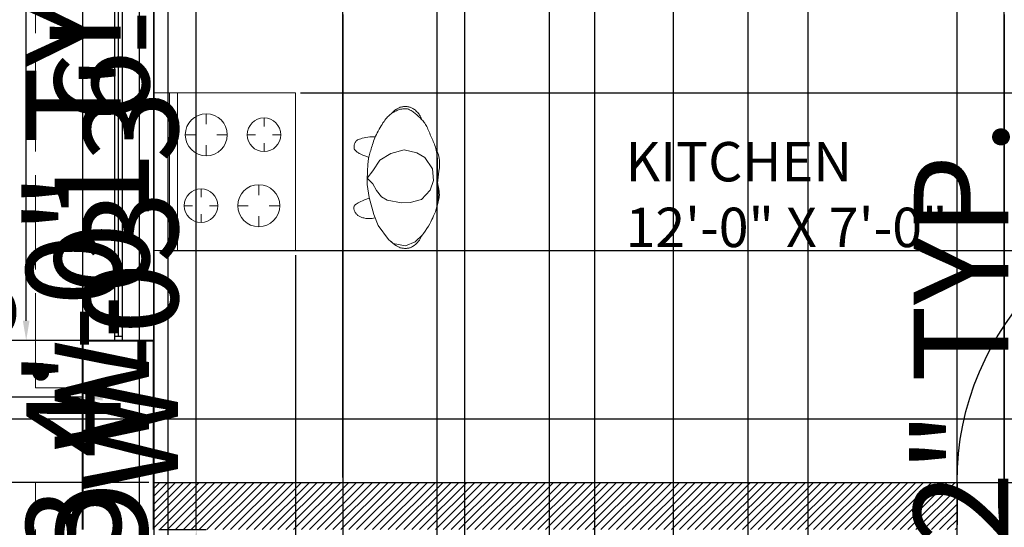
# Model space of a CAD drawing. Units: inches. Extents: x 2386 to 3029, y 792 to 1465.
# Tile 7 of 12: x 2463 to 2588, y 1140 to 1205. Entities that reach past the tile are written whole.
import ezdxf

# ---------------------------------------------------------------- set-up
doc = ezdxf.new("R2010")
doc.units = ezdxf.units.IN
doc.linetypes.add('ACAD_ISO02W100', pattern=[15, 12, -3])
for name, color, linetype, lineweight in [('A-AREA-IDEN', 4, 'Continuous', 25), ('A-DIMS', 1, 'Continuous', 18), ('A-DOOR', 2, 'Continuous', 25), ('A-EQPM', 8, 'Continuous', 18), ('A-FLOR-CASE', 6, 'Continuous', 18), ('A-FURN-ENTG', 8, 'Continuous', 13), ('A-WALL-EXT', 7, 'Continuous', 40), ('A-WALL-INT', 9, 'Continuous', 30), ('A-WALL-PATT', 9, 'Continuous', 13), ('A-WINDOW', 4, 'Continuous', 25), ('A-WINDOW-OVHD', 4, 'ACAD_ISO02W100', 18)]:
    doc.layers.add(name, color=color, linetype=linetype, lineweight=lineweight)
doc.styles.add('ATT', font='romans.shx')
doc.styles.get("Standard").update_dxf_attribs({"font": 'arial.ttf'})
doc.dimstyles.new('ISO-25', dxfattribs={"dimtxt": 12, "dimasz": 2.5, "dimexe": 1.25, "dimexo": 0.625, "dimtad": 1, "dimlunit": 4, "dimtxsty": 'Standard', "dimcen": 2.5, "dimadec": 0, "dimazin": 0, "dimtfac": 1, "dimtmove": 0, "dimatfit": 3, "dimfxl": 1, "dimarcsym": 0})

# ---------------------------------------------------------------- blocks, each defined once
blk = doc.blocks.new('*U14')
for p, q in [((-40, 0), (-40, 6)), ((0, 0), (0, 6))]:
    blk.add_line(p, q)
blk.add_lwpolyline([(0, 0), (0, -40), (-1.75, -40), (-1.75, 0)], close=True)
blk.add_arc((0, 0), 40, 180, 270)
blk = doc.blocks.new('11PRNG01')
at = {"color": 0, "linetype": 'ByBlock'}
for p, q in [((0, 30), (27, 30)), ((0, 0), (0, 30)), ((3, 0), (3, 30)), ((4.5, 0), (4.5, 30)), ((27, 30), (27, 0)), ((10, 26), (10, 24)), ((21, 25.2), (21, 23.6)), ((6, 22), (8, 22)), ((14, 22), (12, 22)), ((17.8, 22), (19.4, 22)), ((24.2, 22), (22.6, 22)), ((10, 18), (10, 20)), ((21, 18.8), (21, 20.4)), ((9, 11.7), (9, 10.1)), ((20, 12.5), (20, 10.5)), ((5.8, 8.5), (7.4, 8.5)), ((12.2, 8.5), (10.6, 8.5)), ((16, 8.5), (18, 8.5)), ((24, 8.5), (22, 8.5)), ((9, 5.3), (9, 6.9)), ((20, 4.5), (20, 6.5)), ((27, 0), (0, 0))]:
    blk.add_line(p, q, dxfattribs=at)
for centre, radius in [((10, 22), 4), ((21, 22), 3.2), ((9, 8.5), 3.2), ((20, 8.5), 4)]:
    blk.add_circle(centre, radius, dxfattribs=at)
at = {"color": 0, "linetype": 'ByBlock', "style": 'ATT'}
for tag, p, flags in [('ITEM', (0, -11), 3), ('ROOM_NUMBER', (0, -20), 1), ('DEPTH', (0, -29), 3), ('WIDTH', (0, -38), 3)]:
    blk.add_attdef(tag, p, '', height=6, dxfattribs=dict(at, flags=flags))
blk = doc.blocks.new('PERSON-STANDING-PLAN')
for p, q in [((4.11, 9.95), (4.28, 10.02)), ((4.28, 10.02), (4.45, 10.1)), ((4.45, 10.1), (4.62, 10.18)), ((4.62, 10.18), (4.79, 10.25)), ((4.79, 10.25), (4.96, 10.31)), ((4.96, 10.31), (5.14, 10.38)), ((5.14, 10.38), (5.33, 10.43)), ((5.33, 10.43), (5.53, 10.48)), ((5.48, 10.5), (5.36, 10.44)), ((5.69, 10.59), (5.48, 10.5)), ((5.53, 10.48), (5.74, 10.51)), ((5.91, 10.67), (5.69, 10.59)), ((5.74, 10.51), (5.95, 10.55)), ((6.13, 10.74), (5.91, 10.67)), ((5.95, 10.55), (6.17, 10.57)), ((6.35, 10.79), (6.13, 10.74)), ((6.17, 10.57), (6.39, 10.59)), ((6.57, 10.84), (6.35, 10.79)), ((6.39, 10.59), (6.61, 10.61)), ((6.79, 10.87), (6.57, 10.84)), ((6.61, 10.61), (6.83, 10.62)), ((6.99, 10.89), (6.79, 10.87)), ((6.83, 10.62), (7.05, 10.63)), ((7.18, 10.9), (6.99, 10.89)), ((7.05, 10.63), (7.26, 10.64)), ((7.38, 10.9), (7.18, 10.9)), ((7.26, 10.64), (7.47, 10.65)), ((7.57, 10.88), (7.38, 10.9)), ((7.47, 10.65), (7.68, 10.65)), ((7.78, 10.87), (7.57, 10.88)), ((7.68, 10.65), (7.87, 10.65)), ((7.99, 10.84), (7.78, 10.87)), ((7.87, 10.65), (8.06, 10.65)), ((9.39, 10.13), (7.91, 9.98)), ((8.22, 10.82), (7.99, 10.84)), ((8.06, 10.65), (8.23, 10.65)), ((9.71, 10.64), (8.22, 10.82)), ((8.23, 10.65), (8.39, 10.65)), ((8.39, 10.65), (8.54, 10.64)), ((8.54, 10.64), (8.67, 10.64)), ((8.67, 10.64), (8.78, 10.63)), ((8.78, 10.63), (8.89, 10.62)), ((8.89, 10.62), (8.98, 10.61)), ((8.98, 10.61), (9.08, 10.6)), ((9.08, 10.6), (9.16, 10.59)), ((9.16, 10.59), (9.25, 10.59)), ((9.25, 10.59), (9.35, 10.59)), ((9.35, 10.59), (9.44, 10.59)), ((10.63, 9.72), (9.39, 10.13)), ((9.44, 10.59), (9.55, 10.6)), ((9.55, 10.6), (9.66, 10.61)), ((9.9, 10.69), (9.56, 10.61)), ((9.66, 10.61), (9.78, 10.62)), ((9.78, 10.62), (9.9, 10.63)), ((10.22, 10.76), (9.9, 10.69)), ((9.9, 10.63), (10.03, 10.64)), ((10.03, 10.64), (10.16, 10.66)), ((10.16, 10.66), (10.3, 10.67)), ((10.5, 10.81), (10.22, 10.76)), ((10.3, 10.67), (10.45, 10.68)), ((10.45, 10.68), (10.61, 10.7)), ((10.76, 10.84), (10.5, 10.81)), ((10.61, 10.7), (10.76, 10.71)), ((10.99, 10.86), (10.76, 10.84)), ((10.76, 10.71), (10.92, 10.71)), ((10.92, 10.71), (11.09, 10.72)), ((11.2, 10.87), (10.99, 10.86)), ((11.09, 10.72), (11.25, 10.72)), ((11.4, 10.86), (11.2, 10.87)), ((11.25, 10.72), (11.41, 10.72)), ((11.58, 10.84), (11.4, 10.86)), ((11.41, 10.72), (11.57, 10.71)), ((11.57, 10.71), (11.73, 10.7)), ((11.76, 10.81), (11.58, 10.84)), ((11.73, 10.7), (11.89, 10.68)), ((11.93, 10.77), (11.76, 10.81)), ((11.89, 10.68), (12.04, 10.67)), ((12.11, 10.73), (11.93, 10.77)), ((12.04, 10.67), (12.19, 10.64)), ((12.29, 10.67), (12.11, 10.73)), ((12.19, 10.64), (12.34, 10.62)), ((12.48, 10.61), (12.29, 10.67)), ((12.34, 10.62), (12.48, 10.59)), ((12.68, 10.55), (12.48, 10.61)), ((12.48, 10.59), (12.63, 10.56)), ((12.63, 10.56), (12.77, 10.53)), ((12.91, 10.49), (12.68, 10.55)), ((12.77, 10.53), (12.91, 10.49)), ((12.91, 10.49), (13.05, 10.45)), ((13.17, 10.43), (12.91, 10.49)), ((13.05, 10.45), (13.2, 10.41)), ((13.2, 10.41), (13.35, 10.36)), ((13.35, 10.36), (13.51, 10.3)), ((13.51, 10.3), (13.69, 10.22)), ((13.69, 10.22), (13.89, 10.14)), ((13.89, 10.14), (14.11, 10.04)), ((14.11, 10.04), (14.35, 9.93)), ((1.69, 8.66), (1.79, 8.76)), ((1.79, 8.76), (1.9, 8.85)), ((1.9, 8.85), (2.01, 8.94)), ((2.01, 8.94), (2.13, 9.02)), ((2.13, 9.02), (2.26, 9.11)), ((2.26, 9.11), (2.39, 9.19)), ((2.39, 9.19), (2.54, 9.27)), ((2.54, 9.27), (2.7, 9.35)), ((2.7, 9.35), (2.86, 9.42)), ((2.86, 9.42), (3.04, 9.5)), ((3.04, 9.5), (3.21, 9.57)), ((3.21, 9.57), (3.39, 9.65)), ((3.39, 9.65), (3.58, 9.72)), ((3.58, 9.72), (3.76, 9.79)), ((3.76, 9.79), (3.94, 9.87)), ((3.94, 9.87), (4.11, 9.95)), ((6.48, 9.01), (5.88, 8.02)), ((7.91, 9.98), (6.48, 9.01)), ((11.79, 8.58), (10.63, 9.72)), ((14.35, 9.93), (14.61, 9.79)), ((14.61, 9.79), (14.89, 9.64)), ((14.89, 9.64), (15.18, 9.47)), ((15.18, 9.47), (15.49, 9.28)), ((15.49, 9.28), (15.8, 9.07)), ((15.8, 9.07), (16.12, 8.84)), ((16.12, 8.84), (16.44, 8.59)), ((0.25, 7.51), (0.2, 7.42)), ((0.32, 7.61), (0.25, 7.51)), ((0.39, 7.71), (0.32, 7.61)), ((0.48, 7.82), (0.39, 7.71)), ((0.57, 7.92), (0.48, 7.82)), ((0.67, 8.02), (0.57, 7.92)), ((0.6, 7.41), (0.68, 7.53)), ((0.77, 8.12), (0.67, 8.02)), ((0.68, 7.53), (0.76, 7.64)), ((0.76, 7.64), (0.85, 7.75)), ((0.87, 8.21), (0.77, 8.12)), ((0.85, 7.75), (0.94, 7.85)), ((0.97, 8.29), (0.87, 8.21)), ((0.94, 7.85), (1.03, 7.96)), ((1.08, 8.36), (0.97, 8.29)), ((1.03, 7.96), (1.12, 8.07)), ((1.17, 8.42), (1.08, 8.36)), ((1.12, 8.07), (1.21, 8.17)), ((1.26, 8.47), (1.17, 8.42)), ((1.21, 8.17), (1.3, 8.27)), ((1.35, 8.51), (1.26, 8.47)), ((1.3, 8.27), (1.39, 8.37)), ((1.43, 8.54), (1.35, 8.51)), ((1.39, 8.37), (1.49, 8.47)), ((1.49, 8.56), (1.43, 8.54)), ((1.55, 8.58), (1.49, 8.56)), ((1.49, 8.47), (1.59, 8.57)), ((1.59, 8.59), (1.55, 8.58)), ((1.59, 8.57), (1.69, 8.66)), ((1.62, 8.6), (1.59, 8.59)), ((5.88, 8.02), (5.48, 6.38)), ((12.18, 7.14), (11.79, 8.58)), ((16.26, 8.74), (17.17, 7.78)), ((16.44, 8.59), (16.61, 8.53)), ((16.61, 8.53), (16.77, 8.45)), ((16.77, 8.45), (16.94, 8.35)), ((16.94, 8.35), (17.1, 8.23)), ((17.1, 8.23), (17.25, 8.1)), ((17.17, 7.78), (17.68, 6.58)), ((17.25, 8.1), (17.38, 7.96)), ((17.38, 7.96), (17.51, 7.82)), ((17.51, 7.82), (17.61, 7.69)), ((17.61, 7.69), (17.7, 7.56)), ((17.7, 7.56), (17.78, 7.45)), ((0.01, 6.79), (0, 6.7)), ((0, 6.7), (0, 6.61)), ((0, 6.61), (0, 6.52)), ((0, 6.52), (0, 6.42)), ((0, 6.42), (0.01, 6.33)), ((0.02, 6.88), (0.01, 6.79)), ((0.01, 6.33), (0.02, 6.22)), ((0.04, 6.97), (0.02, 6.88)), ((0.06, 7.06), (0.04, 6.97)), ((0.08, 7.15), (0.06, 7.06)), ((0.11, 7.23), (0.08, 7.15)), ((0.15, 7.32), (0.11, 7.23)), ((0.2, 7.42), (0.15, 7.32)), ((0.28, 6.52), (0.29, 6.66)), ((0.29, 6.38), (0.28, 6.52)), ((0.29, 6.66), (0.31, 6.8)), ((0.3, 6.24), (0.29, 6.38)), ((0.31, 6.8), (0.35, 6.93)), ((0.35, 6.93), (0.4, 7.06)), ((0.4, 7.06), (0.46, 7.18)), ((0.46, 7.18), (0.52, 7.3)), ((0.52, 7.3), (0.6, 7.41)), ((5.48, 6.38), (5.95, 4.72)), ((12.22, 6.07), (12.18, 7.14)), ((17.68, 6.58), (17.36, 5.01)), ((17.78, 7.45), (17.84, 7.34)), ((17.84, 7.34), (17.88, 7.24)), ((17.88, 7.24), (17.92, 7.15)), ((17.92, 7.15), (17.95, 7.06)), ((17.95, 7.06), (17.97, 6.97)), ((17.97, 6.97), (17.98, 6.88)), ((17.98, 6.88), (17.99, 6.79)), ((17.99, 6.33), (17.98, 6.22)), ((17.99, 6.79), (18, 6.7)), ((18, 6.42), (17.99, 6.33)), ((18, 6.7), (18.01, 6.61)), ((18.01, 6.52), (18, 6.42)), ((18.01, 6.61), (18.01, 6.52)), ((0.02, 6.22), (0.04, 6.12)), ((0.04, 6.12), (0.06, 6)), ((0.06, 6), (0.1, 5.88)), ((0.1, 5.88), (0.15, 5.75)), ((0.15, 5.75), (0.23, 5.6)), ((0.23, 5.6), (0.33, 5.43)), ((0.32, 6.09), (0.3, 6.24)), ((0.35, 5.95), (0.32, 6.09)), ((0.33, 5.43), (0.48, 5.23)), ((0.39, 5.81), (0.35, 5.95)), ((0.43, 5.68), (0.39, 5.81)), ((0.48, 5.55), (0.43, 5.68)), ((0.53, 5.42), (0.48, 5.55)), ((0.48, 5.23), (0.67, 5.01)), ((0.58, 5.3), (0.53, 5.42)), ((0.64, 5.19), (0.58, 5.3)), ((0.7, 5.07), (0.64, 5.19)), ((0.67, 5.01), (0.91, 4.75)), ((0.77, 4.96), (0.7, 5.07)), ((11.9, 4.25), (12.22, 6.07)), ((17.36, 5.01), (16.88, 4.4)), ((17.54, 5.23), (17.37, 5)), ((17.68, 5.42), (17.54, 5.23)), ((17.78, 5.6), (17.68, 5.42)), ((17.86, 5.75), (17.78, 5.6)), ((17.91, 5.88), (17.86, 5.75)), ((17.94, 6), (17.91, 5.88)), ((17.96, 6.12), (17.94, 6)), ((17.98, 6.22), (17.96, 6.12)), ((0.85, 4.85), (0.77, 4.96)), ((0.93, 4.74), (0.85, 4.85)), ((1.01, 4.63), (0.93, 4.74)), ((1.1, 4.52), (1.01, 4.63)), ((1.21, 4.41), (1.1, 4.52)), ((1.32, 4.3), (1.21, 4.41)), ((1.44, 4.19), (1.32, 4.3)), ((1.57, 4.08), (1.44, 4.19)), ((1.72, 3.96), (1.57, 4.08)), ((1.88, 3.84), (1.72, 3.96)), ((2.06, 3.71), (1.88, 3.84)), ((5.95, 4.72), (6.81, 3.29)), ((11.44, 3.53), (11.9, 4.25)), ((16.88, 4.4), (15.08, 3.08)), ((17.37, 5), (17.14, 4.74)), ((2.26, 3.59), (2.06, 3.71)), ((2.46, 3.46), (2.26, 3.59)), ((2.67, 3.34), (2.46, 3.46)), ((2.89, 3.21), (2.67, 3.34)), ((3.11, 3.09), (2.89, 3.21)), ((3.33, 2.98), (3.11, 3.09)), ((3.56, 2.87), (3.33, 2.98)), ((3.77, 2.77), (3.56, 2.87)), ((3.99, 2.68), (3.77, 2.77)), ((3.86, 2.7), (3.84, 2.5)), ((4.2, 2.6), (3.99, 2.68)), ((4.4, 2.52), (4.2, 2.6)), ((4.6, 2.45), (4.4, 2.52)), ((6.81, 3.29), (8.17, 2.41)), ((9.82, 2.41), (10.66, 2.88)), ((10.66, 2.88), (11.44, 3.53)), ((13.68, 2.54), (11.53, 1.95)), ((15.08, 3.08), (13.68, 2.54)), ((14.17, 2.51), (14.14, 2.7)), ((14.19, 2.34), (14.17, 2.51)), ((3.84, 2.5), (3.84, 2.27)), ((3.84, 2.27), (3.86, 2.03)), ((3.86, 2.03), (3.89, 1.79)), ((3.89, 1.79), (3.93, 1.54)), ((3.93, 1.54), (3.98, 1.3)), ((3.98, 1.3), (4.03, 1.08)), ((4.8, 2.38), (4.6, 2.45)), ((5, 2.32), (4.8, 2.38)), ((5.19, 2.26), (5, 2.32)), ((5.38, 2.2), (5.19, 2.26)), ((5.56, 2.15), (5.38, 2.2)), ((5.74, 2.09), (5.56, 2.15)), ((5.92, 2.05), (5.74, 2.09)), ((6.09, 2), (5.92, 2.05)), ((6.25, 1.96), (6.09, 2)), ((6.17, 1.17), (6.26, 1.39)), ((6.41, 1.92), (6.25, 1.96)), ((6.26, 1.39), (6.36, 1.65)), ((6.36, 1.65), (6.46, 1.91)), ((6.55, 1.89), (6.41, 1.92)), ((6.7, 1.86), (6.55, 1.89)), ((6.85, 1.83), (6.7, 1.86)), ((7.04, 1.81), (6.85, 1.83)), ((7.27, 1.79), (7.04, 1.81)), ((7.57, 1.77), (7.27, 1.79)), ((7.97, 1.75), (7.57, 1.77)), ((8.47, 1.73), (7.97, 1.75)), ((8.17, 2.41), (9.1, 1.71)), ((9.1, 1.71), (8.47, 1.73)), ((9.1, 1.71), (9.82, 2.41)), ((9.89, 1.71), (9.1, 1.71)), ((11.53, 1.95), (9.89, 1.71)), ((11.63, 1.91), (11.75, 1.61)), ((11.75, 1.61), (11.85, 1.34)), ((11.85, 1.34), (11.95, 1.1)), ((14.12, 1.15), (14.14, 1.27)), ((14.14, 1.27), (14.17, 1.4)), ((14.17, 1.4), (14.19, 1.54)), ((14.2, 2.16), (14.19, 2.34)), ((14.19, 1.54), (14.2, 1.68)), ((14.21, 1.99), (14.2, 2.16)), ((14.2, 1.68), (14.21, 1.83)), ((14.21, 1.83), (14.21, 1.99)), ((4.03, 1.08), (4.09, 0.89)), ((4.09, 0.89), (4.14, 0.73)), ((4.14, 0.73), (4.19, 0.59)), ((4.19, 0.59), (4.24, 0.49)), ((4.24, 0.49), (4.29, 0.4)), ((4.29, 0.4), (4.34, 0.34)), ((4.34, 0.34), (4.39, 0.28)), ((4.39, 0.28), (4.45, 0.24)), ((4.45, 0.24), (4.51, 0.2)), ((4.51, 0.2), (4.57, 0.17)), ((4.57, 0.17), (4.64, 0.14)), ((4.64, 0.14), (4.72, 0.11)), ((4.72, 0.11), (4.79, 0.09)), ((4.79, 0.09), (4.86, 0.07)), ((4.86, 0.07), (4.93, 0.05)), ((4.93, 0.05), (5, 0.04)), ((5, 0.04), (5.07, 0.03)), ((5.07, 0.03), (5.13, 0.03)), ((5.13, 0.03), (5.19, 0.03)), ((5.19, 0.03), (5.24, 0.03)), ((5.24, 0.03), (5.29, 0.04)), ((5.29, 0.04), (5.34, 0.05)), ((5.34, 0.05), (5.39, 0.06)), ((5.39, 0.06), (5.43, 0.08)), ((5.43, 0.08), (5.47, 0.11)), ((5.47, 0.11), (5.51, 0.13)), ((5.51, 0.13), (5.55, 0.16)), ((5.55, 0.16), (5.59, 0.2)), ((5.59, 0.2), (5.63, 0.24)), ((5.63, 0.24), (5.68, 0.29)), ((5.68, 0.29), (5.72, 0.35)), ((5.72, 0.35), (5.77, 0.42)), ((5.77, 0.42), (5.82, 0.5)), ((5.82, 0.5), (5.88, 0.59)), ((5.88, 0.59), (5.94, 0.7)), ((5.94, 0.7), (6.01, 0.83)), ((6.01, 0.83), (6.09, 0.99)), ((6.09, 0.99), (6.17, 1.17)), ((11.95, 1.1), (12.05, 0.89)), ((12.05, 0.89), (12.13, 0.71)), ((12.13, 0.71), (12.22, 0.55)), ((12.22, 0.55), (12.29, 0.41)), ((12.29, 0.41), (12.37, 0.3)), ((12.37, 0.3), (12.44, 0.21)), ((12.44, 0.21), (12.51, 0.14)), ((12.51, 0.14), (12.58, 0.08)), ((12.58, 0.08), (12.64, 0.04)), ((12.64, 0.04), (12.71, 0.02)), ((12.71, 0.02), (12.77, 0)), ((12.77, 0), (12.84, 0)), ((12.84, 0), (12.9, 0)), ((12.9, 0), (12.97, 0.01)), ((12.97, 0.01), (13.03, 0.02)), ((13.03, 0.02), (13.1, 0.04)), ((13.1, 0.04), (13.17, 0.06)), ((13.17, 0.06), (13.24, 0.09)), ((13.24, 0.09), (13.3, 0.12)), ((13.3, 0.12), (13.37, 0.15)), ((13.37, 0.15), (13.43, 0.18)), ((13.43, 0.18), (13.49, 0.22)), ((13.49, 0.22), (13.55, 0.26)), ((13.55, 0.26), (13.61, 0.31)), ((13.61, 0.31), (13.67, 0.35)), ((13.67, 0.35), (13.72, 0.41)), ((13.72, 0.41), (13.77, 0.47)), ((13.77, 0.47), (13.82, 0.53)), ((13.82, 0.53), (13.87, 0.6)), ((13.87, 0.6), (13.92, 0.67)), ((13.92, 0.67), (13.96, 0.75)), ((13.96, 0.75), (14.01, 0.84)), ((14.01, 0.84), (14.05, 0.94)), ((14.05, 0.94), (14.08, 1.04)), ((14.08, 1.04), (14.12, 1.15))]:
    blk.add_line(p, q)
blk = doc.blocks.new('WINDOW-48IN')
for p, q in [((0, 9), (48, 9)), ((0, 0), (0, 9)), ((48, 9), (48, 0)), ((48, 5), (0, 5)), ((48, 4), (0, 4)), ((0.5, 4), (0.5, 5)), ((47.5, 4.5), (0.5, 4.5)), ((47.5, 5), (47.5, 4)), ((48, 0), (0, 0))]:
    blk.add_line(p, q)
blk = doc.blocks.new('WINDOW-HOOD-48IN')
for p, q in [((0, 0), (0, 6)), ((60, 6), (60, 0)), ((60, 0), (0, 0))]:
    blk.add_line(p, q)
blk = doc.blocks.new('WINDOW-HOOD-36IN')
for p, q in [((0, 0), (0, 48)), ((0, 48), (6, 48)), ((6, 0), (0, 0))]:
    blk.add_line(p, q)
blk = doc.blocks.new('*D38')
at = {"layer": 'A-DIMS', "color": 0, "lineweight": -2, "transparency": 16777216}
for p, q in [((2471.82, 1342.95), (2483.24, 1342.95)), ((2481.99, 1340.45), (2481.99, 1273.45)), ((2471.82, 1270.95), (2483.24, 1270.95)), ((2481.99, 1270.95), (2481.99, 1095.04))]:
    blk.add_line(p, q, dxfattribs=at)
at = {"layer": 'A-DIMS', "color": 0, "transparency": 16777216}
for points in [[(2481.57, 1340.45), (2482.41, 1340.45), (2481.99, 1342.95)], [(2481.57, 1273.45), (2482.41, 1273.45), (2481.99, 1270.95)]]:
    blk.add_solid(points, dxfattribs=at)
at = {"layer": 'Defpoints', "color": 0, "transparency": 16777216}
for p in [(2471.19, 1342.95), (2471.19, 1270.95), (2481.99, 1270.95)]:
    blk.add_point(p, dxfattribs=at)
at = {"layer": 'A-DIMS', "color": 0, "transparency": 16777216, "insert": (2475.16, 1181.74), "char_height": 12, "attachment_point": 5, "rotation": 90}
blk.add_mtext('HOOD W-01 6\'-0" TYP.', dxfattribs=at)
blk = doc.blocks.new('*D40')
at = {"layer": 'A-DIMS', "color": 0, "lineweight": -2, "transparency": 16777216}
for p, q in [((2463.99, 1211.95), (2463.99, 1334.04)), ((2470.57, 1211.95), (2462.74, 1211.95)), ((2463.99, 1166.45), (2463.99, 1209.45)), ((2470.57, 1163.95), (2462.74, 1163.95))]:
    blk.add_line(p, q, dxfattribs=at)
at = {"layer": 'A-DIMS', "color": 0, "transparency": 16777216}
for points in [[(2463.57, 1209.45), (2464.41, 1209.45), (2463.99, 1211.95)], [(2463.57, 1166.45), (2464.41, 1166.45), (2463.99, 1163.95)]]:
    blk.add_solid(points, dxfattribs=at)
at = {"layer": 'Defpoints', "color": 0, "transparency": 16777216}
for p in [(2463.99, 1211.95), (2471.19, 1211.95), (2471.19, 1163.95)]:
    blk.add_point(p, dxfattribs=at)
at = {"layer": 'A-DIMS', "color": 0, "transparency": 16777216, "insert": (2457.24, 1274.25), "char_height": 12, "attachment_point": 5, "rotation": 90}
blk.add_mtext('W-02 4\'-0" TYP.', dxfattribs=at)
blk = doc.blocks.new('*D41')
at = {"layer": 'A-DIMS', "color": 0, "lineweight": -2, "transparency": 16777216}
for p, q in [((2471.19, 1163.32), (2471.19, 1155.5)), ((2480.19, 1163.32), (2480.19, 1155.5)), ((2471.19, 1156.75), (2394.29, 1156.75)), ((2477.69, 1156.75), (2473.69, 1156.75))]:
    blk.add_line(p, q, dxfattribs=at)
at = {"layer": 'A-DIMS', "color": 0, "transparency": 16777216}
for points in [[(2473.69, 1157.16), (2473.69, 1156.33), (2471.19, 1156.75)], [(2477.69, 1157.16), (2477.69, 1156.33), (2480.19, 1156.75)]]:
    blk.add_solid(points, dxfattribs=at)
at = {"layer": 'Defpoints', "color": 0, "transparency": 16777216}
for p in [(2471.19, 1163.95), (2480.19, 1163.95), (2471.19, 1156.75)]:
    blk.add_point(p, dxfattribs=at)
at = {"layer": 'A-DIMS', "color": 0, "transparency": 16777216, "insert": (2431.49, 1163.5), "char_height": 12, "attachment_point": 5}
blk.add_mtext('0\'-9" TYP.', dxfattribs=at)
blk = doc.blocks.new('*D44')
at = {"layer": 'A-DIMS', "color": 0, "lineweight": -2, "transparency": 16777216}
for p, q in [((2485.59, 1139.95), (2485.59, 1262.04)), ((2480.82, 1139.95), (2486.84, 1139.95)), ((2485.59, 1106.45), (2485.59, 1137.45)), ((2480.82, 1103.95), (2486.84, 1103.95))]:
    blk.add_line(p, q, dxfattribs=at)
at = {"layer": 'A-DIMS', "color": 0, "transparency": 16777216}
for points in [[(2485.17, 1137.45), (2486.01, 1137.45), (2485.59, 1139.95)], [(2485.17, 1106.45), (2486.01, 1106.45), (2485.59, 1103.95)]]:
    blk.add_solid(points, dxfattribs=at)
at = {"layer": 'Defpoints', "color": 0, "transparency": 16777216}
for p in [(2480.19, 1139.95), (2485.59, 1139.95), (2480.19, 1103.95)]:
    blk.add_point(p, dxfattribs=at)
at = {"layer": 'A-DIMS', "color": 0, "transparency": 16777216, "insert": (2478.83, 1202.25), "char_height": 12, "attachment_point": 5, "rotation": 90}
blk.add_mtext('W-03 3\'-0" TYP.', dxfattribs=at)
blk = doc.blocks.new('*D46')
at = {"layer": 'A-DIMS', "color": 0, "lineweight": -2, "transparency": 16777216}
for p, q in [((2478.39, 1049.95), (2478.39, 1225.86)), ((2471.82, 1049.95), (2479.64, 1049.95)), ((2478.39, 1004.45), (2478.39, 1047.45)), ((2471.82, 1001.95), (2479.64, 1001.95))]:
    blk.add_line(p, q, dxfattribs=at)
at = {"layer": 'A-DIMS', "color": 0, "transparency": 16777216}
for points in [[(2477.97, 1047.45), (2478.81, 1047.45), (2478.39, 1049.95)], [(2477.97, 1004.45), (2478.81, 1004.45), (2478.39, 1001.95)]]:
    blk.add_solid(points, dxfattribs=at)
at = {"layer": 'Defpoints', "color": 0, "transparency": 16777216}
for p in [(2471.19, 1049.95), (2478.39, 1049.95), (2471.19, 1001.95)]:
    blk.add_point(p, dxfattribs=at)
at = {"layer": 'A-DIMS', "color": 0, "transparency": 16777216, "insert": (2471.55, 1139.15), "char_height": 12, "attachment_point": 5, "rotation": 90}
blk.add_mtext('HOOD W-03 4\'-0" TYP.', dxfattribs=at)
blk = doc.blocks.new('*D52')
at = {"layer": 'A-DIMS', "color": 0, "lineweight": -2, "transparency": 16777216}
for p, q in [((2595.33, 1229.95), (2589.83, 1229.95)), ((2591.08, 1227.45), (2591.08, 1199.96)), ((2595.33, 1197.46), (2589.83, 1197.46)), ((2591.08, 1197.46), (2591.08, 1050.38))]:
    blk.add_line(p, q, dxfattribs=at)
at = {"layer": 'A-DIMS', "color": 0, "transparency": 16777216}
for points in [[(2590.67, 1227.45), (2591.5, 1227.45), (2591.08, 1229.95)], [(2590.67, 1199.96), (2591.5, 1199.96), (2591.08, 1197.46)]]:
    blk.add_solid(points, dxfattribs=at)
at = {"layer": 'Defpoints', "color": 0, "transparency": 16777216}
for p in [(2595.96, 1229.95), (2591.08, 1197.46), (2595.96, 1197.46)]:
    blk.add_point(p, dxfattribs=at)
at = {"layer": 'A-DIMS', "color": 0, "transparency": 16777216, "insert": (2584.25, 1122.67), "char_height": 12, "attachment_point": 5, "rotation": 90}
blk.add_mtext('REF. 2\'-8 1/2" TYP.', dxfattribs=at)
blk = doc.blocks.new('*D57')
at = {"layer": 'A-DIMS', "color": 0, "lineweight": -2, "transparency": 16777216}
for p, q in [((2546.19, 1008.57), (2546.19, 1427.9)), ((2582.19, 1008.57), (2582.19, 1427.9)), ((2548.69, 1426.65), (2579.69, 1426.65))]:
    blk.add_line(p, q, dxfattribs=at)
at = {"layer": 'A-DIMS', "color": 0, "transparency": 16777216}
for points in [[(2548.69, 1427.06), (2548.69, 1426.23), (2546.19, 1426.65)], [(2579.69, 1427.06), (2579.69, 1426.23), (2582.19, 1426.65)]]:
    blk.add_solid(points, dxfattribs=at)
at = {"layer": 'Defpoints', "color": 0, "transparency": 16777216}
for p in [(2582.19, 1426.65), (2546.19, 1007.95), (2582.19, 1007.95)]:
    blk.add_point(p, dxfattribs=at)
at = {"layer": 'A-DIMS', "color": 0, "transparency": 16777216, "insert": (2564.19, 1433.4), "char_height": 12, "attachment_point": 5}
blk.add_mtext('3\'-0"', dxfattribs=at)
blk = doc.blocks.new('*D64')
at = {"layer": 'A-DIMS', "color": 0, "lineweight": -2, "transparency": 16777216}
for p, q in [((2432.49, 1163.95), (2432.49, 1198.47)), ((2479.57, 1163.95), (2431.24, 1163.95)), ((2432.49, 1148.45), (2432.49, 1161.45)), ((2479.57, 1145.95), (2431.24, 1145.95))]:
    blk.add_line(p, q, dxfattribs=at)
at = {"layer": 'A-DIMS', "color": 0, "transparency": 16777216}
for points in [[(2432.07, 1161.45), (2432.91, 1161.45), (2432.49, 1163.95)], [(2432.07, 1148.45), (2432.91, 1148.45), (2432.49, 1145.95)]]:
    blk.add_solid(points, dxfattribs=at)
at = {"layer": 'Defpoints', "color": 0, "transparency": 16777216}
for p in [(2432.49, 1163.95), (2480.19, 1163.95), (2480.19, 1145.95)]:
    blk.add_point(p, dxfattribs=at)
at = {"layer": 'A-DIMS', "color": 0, "transparency": 16777216, "insert": (2425.74, 1182.46), "char_height": 12, "attachment_point": 5, "rotation": 90}
blk.add_mtext('1\'-6"', dxfattribs=at)
blk = doc.blocks.new('*D73')
at = {"layer": 'A-DIMS', "color": 0, "lineweight": -2, "transparency": 16777216}
for p, q in [((2519.68, 889.97), (2519.68, 1427.9)), ((2555.68, 889.97), (2555.68, 1427.9)), ((2522.18, 1426.65), (2553.18, 1426.65))]:
    blk.add_line(p, q, dxfattribs=at)
at = {"layer": 'A-DIMS', "color": 0, "transparency": 16777216}
for points in [[(2522.18, 1427.06), (2522.18, 1426.23), (2519.68, 1426.65)], [(2553.18, 1427.06), (2553.18, 1426.23), (2555.68, 1426.65)]]:
    blk.add_solid(points, dxfattribs=at)
at = {"layer": 'Defpoints', "color": 0, "transparency": 16777216}
for p in [(2555.68, 1426.65), (2519.68, 889.35), (2555.68, 889.35)]:
    blk.add_point(p, dxfattribs=at)
at = {"layer": 'A-DIMS', "color": 0, "transparency": 16777216, "insert": (2537.68, 1433.4), "char_height": 12, "attachment_point": 5}
blk.add_mtext('3\'-0"', dxfattribs=at)
blk = doc.blocks.new('*D75')
at = {"layer": 'A-DIMS', "color": 0, "lineweight": -2, "transparency": 16777216}
for p, q in [((2929.89, 1195.39), (2929.89, 1229.91)), ((2498.82, 1195.39), (2931.14, 1195.39)), ((2929.89, 1177.89), (2929.89, 1192.89)), ((2498.82, 1175.39), (2931.14, 1175.39))]:
    blk.add_line(p, q, dxfattribs=at)
at = {"layer": 'A-DIMS', "color": 0, "transparency": 16777216}
for points in [[(2929.47, 1192.89), (2930.31, 1192.89), (2929.89, 1195.39)], [(2929.47, 1177.89), (2930.31, 1177.89), (2929.89, 1175.39)]]:
    blk.add_solid(points, dxfattribs=at)
at = {"layer": 'Defpoints', "color": 0, "transparency": 16777216}
for p in [(2498.19, 1195.39), (2929.89, 1195.39), (2498.19, 1175.39)]:
    blk.add_point(p, dxfattribs=at)
at = {"layer": 'A-DIMS', "color": 0, "transparency": 16777216, "insert": (2923.14, 1213.9), "char_height": 12, "attachment_point": 5, "rotation": 90}
blk.add_mtext('1\'-8"', dxfattribs=at)
blk = doc.blocks.new('*D76')
at = {"layer": 'A-DIMS', "color": 0, "lineweight": -2, "transparency": 16777216}
for p, q in [((2480.19, 1174.77), (2480.19, 808)), ((2498.19, 1174.77), (2498.19, 808)), ((2482.69, 809.25), (2495.69, 809.25)), ((2498.19, 809.25), (2532.71, 809.25))]:
    blk.add_line(p, q, dxfattribs=at)
at = {"layer": 'A-DIMS', "color": 0, "transparency": 16777216}
for points in [[(2482.69, 809.66), (2482.69, 808.83), (2480.19, 809.25)], [(2495.69, 809.66), (2495.69, 808.83), (2498.19, 809.25)]]:
    blk.add_solid(points, dxfattribs=at)
at = {"layer": 'Defpoints', "color": 0, "transparency": 16777216}
for p in [(2480.19, 1175.39), (2498.19, 1175.39), (2498.19, 809.25)]:
    blk.add_point(p, dxfattribs=at)
at = {"layer": 'A-DIMS', "color": 0, "transparency": 16777216, "insert": (2516.7, 816), "char_height": 12, "attachment_point": 5}
blk.add_mtext('1\'-6"', dxfattribs=at)
blk = doc.blocks.new('*D78')
at = {"layer": 'A-DIMS', "color": 0, "lineweight": -2, "transparency": 16777216}
for p, q in [((2516.19, 1054.57), (2516.19, 1427.9)), ((2536.19, 1044.57), (2536.19, 1427.9)), ((2518.69, 1426.65), (2533.69, 1426.65)), ((2536.19, 1426.65), (2570.71, 1426.65))]:
    blk.add_line(p, q, dxfattribs=at)
at = {"layer": 'A-DIMS', "color": 0, "transparency": 16777216}
for points in [[(2518.69, 1427.06), (2518.69, 1426.23), (2516.19, 1426.65)], [(2533.69, 1427.06), (2533.69, 1426.23), (2536.19, 1426.65)]]:
    blk.add_solid(points, dxfattribs=at)
at = {"layer": 'Defpoints', "color": 0, "transparency": 16777216}
for p in [(2536.19, 1426.65), (2516.19, 1053.95), (2536.19, 1043.95)]:
    blk.add_point(p, dxfattribs=at)
at = {"layer": 'A-DIMS', "color": 0, "transparency": 16777216, "insert": (2554.7, 1433.4), "char_height": 12, "attachment_point": 5}
blk.add_mtext('1\'-8"', dxfattribs=at)
blk = doc.blocks.new('*D81')
at = {"layer": 'A-DIMS', "color": 0, "lineweight": -2, "transparency": 16777216}
for p, q in [((2432.49, 1153.95), (2432.49, 1188.47)), ((2809.57, 1153.95), (2431.24, 1153.95)), ((2432.49, 1138.45), (2432.49, 1151.45)), ((2809.57, 1135.95), (2431.24, 1135.95))]:
    blk.add_line(p, q, dxfattribs=at)
at = {"layer": 'A-DIMS', "color": 0, "transparency": 16777216}
for points in [[(2432.07, 1151.45), (2432.91, 1151.45), (2432.49, 1153.95)], [(2432.07, 1138.45), (2432.91, 1138.45), (2432.49, 1135.95)]]:
    blk.add_solid(points, dxfattribs=at)
at = {"layer": 'Defpoints', "color": 0, "transparency": 16777216}
for p in [(2432.49, 1153.95), (2810.19, 1153.95), (2810.19, 1135.95)]:
    blk.add_point(p, dxfattribs=at)
at = {"layer": 'A-DIMS', "color": 0, "transparency": 16777216, "insert": (2425.74, 1172.46), "char_height": 12, "attachment_point": 5, "rotation": 90}
blk.add_mtext('1\'-6"', dxfattribs=at)
blk = doc.blocks.new('*D94')
at = {"layer": 'A-DIMS', "color": 0, "lineweight": -2, "transparency": 16777216}
for p, q in [((2504.19, 1205.32), (2504.19, 808)), ((2588.19, 1205.32), (2588.19, 808)), ((2506.69, 809.25), (2585.69, 809.25))]:
    blk.add_line(p, q, dxfattribs=at)
at = {"layer": 'A-DIMS', "color": 0, "transparency": 16777216}
for points in [[(2506.69, 809.66), (2506.69, 808.83), (2504.19, 809.25)], [(2585.69, 809.66), (2585.69, 808.83), (2588.19, 809.25)]]:
    blk.add_solid(points, dxfattribs=at)
at = {"layer": 'Defpoints', "color": 0, "transparency": 16777216}
for p in [(2504.19, 1205.95), (2588.19, 1205.95), (2588.19, 809.25)]:
    blk.add_point(p, dxfattribs=at)
at = {"layer": 'A-DIMS', "color": 0, "transparency": 16777216, "insert": (2546.19, 816), "char_height": 12, "attachment_point": 5}
blk.add_mtext('7\'-0"', dxfattribs=at)
blk = doc.blocks.new('*D95')
at = {"layer": 'A-DIMS', "color": 0, "lineweight": -2, "transparency": 16777216}
for p, q in [((2480.19, 1146.57), (2480.19, 1427.9)), ((2504.19, 1146.57), (2504.19, 1427.9)), ((2482.69, 1426.65), (2501.69, 1426.65)), ((2504.19, 1426.65), (2540.04, 1426.65))]:
    blk.add_line(p, q, dxfattribs=at)
at = {"layer": 'A-DIMS', "color": 0, "transparency": 16777216}
for points in [[(2482.69, 1427.06), (2482.69, 1426.23), (2480.19, 1426.65)], [(2501.69, 1427.06), (2501.69, 1426.23), (2504.19, 1426.65)]]:
    blk.add_solid(points, dxfattribs=at)
at = {"layer": 'Defpoints', "color": 0, "transparency": 16777216}
for p in [(2504.19, 1426.65), (2480.19, 1145.95), (2504.19, 1145.95)]:
    blk.add_point(p, dxfattribs=at)
at = {"layer": 'A-DIMS', "color": 0, "transparency": 16777216, "insert": (2523.37, 1433.4), "char_height": 12, "attachment_point": 5}
blk.add_mtext('2\'-0"', dxfattribs=at)
blk = doc.blocks.new('*D96')
at = {"layer": 'A-DIMS', "color": 0, "lineweight": -2, "transparency": 16777216}
for p, q in [((2516.19, 893.57), (2516.19, 1427.9)), ((2588.19, 893.57), (2588.19, 1427.9)), ((2518.69, 1426.65), (2585.69, 1426.65))]:
    blk.add_line(p, q, dxfattribs=at)
at = {"layer": 'A-DIMS', "color": 0, "transparency": 16777216}
for points in [[(2518.69, 1427.06), (2518.69, 1426.23), (2516.19, 1426.65)], [(2585.69, 1427.06), (2585.69, 1426.23), (2588.19, 1426.65)]]:
    blk.add_solid(points, dxfattribs=at)
at = {"layer": 'Defpoints', "color": 0, "transparency": 16777216}
for p in [(2588.19, 1426.65), (2516.19, 892.95), (2588.19, 892.95)]:
    blk.add_point(p, dxfattribs=at)
at = {"layer": 'A-DIMS', "color": 0, "transparency": 16777216, "insert": (2552.19, 1433.4), "char_height": 12, "attachment_point": 5}
blk.add_mtext('6\'-0"', dxfattribs=at)
blk = doc.blocks.new('*D99')
at = {"layer": 'A-DIMS', "color": 0, "lineweight": -2, "transparency": 16777216}
for p, q in [((2530.41, 1210.29), (2530.41, 808)), ((2563.26, 1210.63), (2563.26, 808)), ((2532.91, 809.25), (2560.76, 809.25)), ((2563.26, 809.25), (2599.11, 809.25))]:
    blk.add_line(p, q, dxfattribs=at)
at = {"layer": 'A-DIMS', "color": 0, "transparency": 16777216}
for points in [[(2532.91, 809.66), (2532.91, 808.83), (2530.41, 809.25)], [(2560.76, 809.66), (2560.76, 808.83), (2563.26, 809.25)]]:
    blk.add_solid(points, dxfattribs=at)
at = {"layer": 'Defpoints', "color": 0, "transparency": 16777216}
for p in [(2530.41, 1210.91), (2563.26, 1211.26), (2563.26, 809.25)]:
    blk.add_point(p, dxfattribs=at)
at = {"layer": 'A-DIMS', "color": 0, "transparency": 16777216, "insert": (2582.43, 816), "char_height": 12, "attachment_point": 5}
blk.add_mtext('2\'-9"', dxfattribs=at)
blk = doc.blocks.new('*D100')
at = {"layer": 'A-DIMS', "color": 0, "lineweight": -2, "transparency": 16777216}
for p, q in [((2562.86, 1228.59), (2931.14, 1228.59)), ((2929.89, 1226.09), (2929.89, 1212.84)), ((2563.05, 1210.34), (2931.14, 1210.34)), ((2929.89, 1210.34), (2929.89, 1147.86))]:
    blk.add_line(p, q, dxfattribs=at)
at = {"layer": 'A-DIMS', "color": 0, "transparency": 16777216}
for points in [[(2929.47, 1226.09), (2930.31, 1226.09), (2929.89, 1228.59)], [(2929.47, 1212.84), (2930.31, 1212.84), (2929.89, 1210.34)]]:
    blk.add_solid(points, dxfattribs=at)
at = {"layer": 'Defpoints', "color": 0, "transparency": 16777216}
for p in [(2562.24, 1228.59), (2562.43, 1210.34), (2929.89, 1210.34)]:
    blk.add_point(p, dxfattribs=at)
at = {"layer": 'A-DIMS', "color": 0, "transparency": 16777216, "insert": (2923.06, 1177.85), "char_height": 12, "attachment_point": 5, "rotation": 90}
blk.add_mtext('1\'-6 1/2"', dxfattribs=at)
blk = doc.blocks.new('*D101')
at = {"layer": 'A-DIMS', "color": 0, "lineweight": -2, "transparency": 16777216}
for p, q in [((2929.89, 1175.39), (2929.89, 1239.21)), ((2480.82, 1175.39), (2931.14, 1175.39)), ((2929.89, 1148.45), (2929.89, 1172.89)), ((2480.82, 1145.95), (2931.14, 1145.95))]:
    blk.add_line(p, q, dxfattribs=at)
at = {"layer": 'A-DIMS', "color": 0, "transparency": 16777216}
for points in [[(2929.47, 1172.89), (2930.31, 1172.89), (2929.89, 1175.39)], [(2929.47, 1148.45), (2930.31, 1148.45), (2929.89, 1145.95)]]:
    blk.add_solid(points, dxfattribs=at)
at = {"layer": 'Defpoints', "color": 0, "transparency": 16777216}
for p in [(2480.19, 1175.39), (2929.89, 1175.39), (2480.19, 1145.95)]:
    blk.add_point(p, dxfattribs=at)
at = {"layer": 'A-DIMS', "color": 0, "transparency": 16777216, "insert": (2923.06, 1208.55), "char_height": 12, "attachment_point": 5, "rotation": 90}
blk.add_mtext('2\'-5 1/2"', dxfattribs=at)

msp = doc.modelspace()

# ---------------------------------------------------------------- hatches: boundary and pattern name
at = {"layer": 'A-WALL-PATT'}
h = msp.add_hatch(dxfattribs=at)
h.set_pattern_fill('JIS_WOOD', color=256)
h.paths.add_polyline_path([(2624.19, 1229.948), (2624.19, 1145.948), (2618.19, 1145.948), (2618.19, 1140.548), (2618.19, 1139.948), (2630.19, 1139.948), (2630.19, 1240.948), (2624.19, 1240.948), (2624.19, 1234.948), (2480.19, 1234.948), (2480.19, 1229.948)])
h.paths.add_polyline_path([(2582.19, 1139.948), (2582.19, 1145.948), (2480.19, 1145.948), (2480.19, 1139.948)], flags=17)
h.paths.add_polyline_path([(2480.19, 1007.948), (2480.19, 1001.948), (2546.19, 1001.948), (2546.19, 1007.348), (2546.19, 1007.948)])
h.paths.add_polyline_path([(2594.19, 1007.948), (2582.19, 1007.948), (2582.19, 1001.948), (2588.19, 1001.948), (2588.19, 856.948), (2594.19, 856.948), (2594.19, 914.948), (2606.19, 914.948), (2606.19, 920.948), (2594.19, 920.948)])
h.paths.add_polyline_path([(2738.19, 1015.948), (2882.19, 1015.948), (2882.19, 1021.948), (2738.19, 1021.948), (2738.19, 1111.948), (2732.19, 1111.948), (2732.19, 920.948), (2720.19, 920.948), (2720.19, 914.948), (2732.19, 914.948), (2732.19, 856.948), (2738.19, 856.948)])
h.paths.add_polyline_path([(2660.19, 914.948), (2660.19, 920.948), (2648.19, 920.948), (2648.19, 914.948)])
h.paths.add_polyline_path([(2738.19, 1159.948), (2738.19, 1165.948), (2737.59, 1165.948), (2732.19, 1165.948), (2732.19, 1147.948), (2737.59, 1147.948), (2738.19, 1147.948), (2738.19, 1153.948), (2882.19, 1153.948), (2882.19, 1159.948)])
h.paths.add_polyline_path([(2732.19, 1201.948), (2738.19, 1201.948), (2738.19, 1303.948), (2774.19, 1303.948), (2774.19, 1308.948), (2768.19, 1308.948), (2768.19, 1378.948), (2762.19, 1378.948), (2762.19, 1308.948), (2726.19, 1308.948), (2726.19, 1303.948), (2732.19, 1303.948)])
h.paths.add_polyline_path([(2696.19, 1303.948), (2696.19, 1308.948), (2630.19, 1308.948), (2630.19, 1378.948), (2624.19, 1378.948), (2624.19, 1276.948), (2630.19, 1276.948), (2630.19, 1303.948)])

# ---------------------------------------------------------------- linework, layer by layer
at = {"layer": 'A-FLOR-CASE'}
msp.add_lwpolyline([(2504.19, 1145.948), (2504.19, 1205.948), (2588.19, 1205.948), (2588.19, 1229.948)], dxfattribs=at)
at = {"layer": 'A-WALL-EXT'}
for p, q in [((2471.19, 1163.948), (2480.19, 1163.948)), ((2471.19, 1139.948), (2471.19, 1163.948)), ((2471.19, 1163.948), (2480.19, 1163.948)), ((2480.19, 1139.948), (2480.19, 1163.948))]:
    msp.add_line(p, q, dxfattribs=at)
at = {"layer": 'A-WALL-INT'}
for p in [(2480.19, 1145.948), (2582.19, 1139.948)]:
    msp.add_line(p, (2582.19, 1145.948), dxfattribs=at)

# ---------------------------------------------------------------- block references
at = {"layer": 'A-DOOR', "xscale": -0.9, "yscale": 0.9, "zscale": 0.9, "rotation": 180}
msp.add_blockref('*U14', (2618.19, 1145.948), dxfattribs=at)
at = {"layer": 'A-EQPM', "xscale": 0.6666666666666707, "yscale": 0.6666666666666707, "zscale": 0.6666666666666707}
msp.add_blockref('11PRNG01', (2480.19, 1175.392), dxfattribs=at)
at = {"layer": 'A-FURN-ENTG', "rotation": 269.9999999999584}
msp.add_blockref('PERSON-STANDING-PLAN', (2505.588, 1193.641), dxfattribs=at)
at = {"layer": 'A-WINDOW', "rotation": 89.9999999997146}
msp.add_blockref('WINDOW-48IN', (2480.19, 1163.948), dxfattribs=at)
at = {"layer": 'A-WINDOW-OVHD', "rotation": 269.9999999991061}
msp.add_blockref('WINDOW-HOOD-48IN', (2465.19, 1217.948), dxfattribs=at)
at = {"layer": 'A-WINDOW-OVHD'}
msp.add_blockref('WINDOW-HOOD-36IN', (2465.19, 1097.948), dxfattribs=at)

# ---------------------------------------------------------------- texts
at = {"layer": 'A-AREA-IDEN', "insert": (2540.094, 1189.14), "char_height": 5, "attachment_point": 1}
msp.add_mtext_dynamic_manual_height_columns('KITCHEN \\P12\'-0" X 7\'-0"', width=52.37406, gutter_width=12.5, heights=[0], dxfattribs=at)

# ---------------------------------------------------------------- dimensions: what is measured, and where the dimension line sits
at = {"layer": 'A-DIMS'}
for base, p1, p2, picture, middle in [((2504.19, 1426.648), (2480.19, 1145.948), (2504.19, 1145.948), '*D95', (2523.367, 1433.4)), ((2536.19, 1426.648), (2516.19, 1053.948), (2536.19, 1043.948), '*D78', (2554.7, 1433.4)), ((2588.19, 1426.648), (2516.19, 892.948), (2588.19, 892.948), '*D96', (2552.19, 1433.4)), ((2555.676, 1426.648), (2519.676, 889.348), (2555.676, 889.348), '*D73', (2537.676, 1433.404)), ((2582.19, 1426.648), (2546.19, 1007.948), (2582.19, 1007.948), '*D57', (2564.19, 1433.404)), ((2563.257, 809.248), (2530.413, 1210.915), (2563.257, 1211.257), '*D99', (2582.434, 816)), ((2588.19, 809.248), (2504.19, 1205.948), (2588.19, 1205.948), '*D94', (2546.19, 816)), ((2498.19, 809.248), (2480.19, 1175.392), (2498.19, 1175.392), '*D76', (2516.7, 816))]:
    dim = msp.add_linear_dim(base=base, p1=p1, p2=p2, dimstyle='ISO-25', override={"dimdec": 1, "dimlfac": 1, "dimrnd": 0, "dimzin": 1, "dimdsep": 46, "dimlunit": 4, "dimfrac": 2}, dxfattribs=at)
    dim.commit()
    dim.dimension.update_dxf_attribs({"geometry": picture, "text_midpoint": middle})
for base, p1, p2, angle, text, picture, middle in [((2481.99, 1270.948), (2471.19, 1342.948), (2471.19, 1270.948), 270, 'HOOD W-01 <> TYP.', '*D38', (2475.156, 1181.744)), ((2463.99, 1211.948), (2471.19, 1163.948), (2471.19, 1211.948), 90, 'W-02 <> TYP.', '*D40', (2457.238, 1274.246)), ((2485.59, 1139.948), (2480.19, 1103.948), (2480.19, 1139.948), 90, 'W-03 <> TYP.', '*D44', (2478.834, 1202.246)), ((2591.083, 1197.463), (2595.956, 1229.948), (2595.956, 1197.463), 270, 'REF. <> TYP.', '*D52', (2584.253, 1122.673)), ((2478.39, 1049.948), (2471.19, 1001.948), (2471.19, 1049.948), 90, 'HOOD W-03 <> TYP.', '*D46', (2471.552, 1139.152)), ((2471.19, 1156.748), (2480.19, 1163.948), (2471.19, 1163.948), 180, '<> TYP.', '*D41', (2431.492, 1163.5))]:
    dim = msp.add_linear_dim(base=base, p1=p1, p2=p2, angle=angle, text=text, dimstyle='ISO-25', override={"dimdec": 1, "dimlfac": 1, "dimrnd": 0, "dimzin": 1, "dimdsep": 46, "dimlunit": 4, "dimfrac": 2}, dxfattribs=at)
    dim.commit()
    dim.dimension.update_dxf_attribs({"geometry": picture, "text_midpoint": middle})
for base, p1, p2, picture, middle in [((2929.89, 1175.392), (2480.19, 1145.948), (2480.19, 1175.392), '*D101', (2923.06, 1208.55)), ((2929.89, 1195.392), (2498.19, 1175.392), (2498.19, 1195.392), '*D75', (2923.138, 1213.902)), ((2929.89, 1210.342), (2562.236, 1228.595), (2562.425, 1210.342), '*D100', (2923.06, 1177.852)), ((2432.49, 1163.948), (2480.19, 1145.948), (2480.19, 1163.948), '*D64', (2425.738, 1182.458)), ((2432.49, 1153.948), (2810.19, 1135.948), (2810.19, 1153.948), '*D81', (2425.738, 1172.458))]:
    dim = msp.add_linear_dim(base=base, p1=p1, p2=p2, angle=90, dimstyle='ISO-25', override={"dimdec": 1, "dimlfac": 1, "dimrnd": 0, "dimzin": 1, "dimdsep": 46, "dimlunit": 4, "dimfrac": 2}, dxfattribs=at)
    dim.commit()
    dim.dimension.update_dxf_attribs({"geometry": picture, "text_midpoint": middle})

doc.saveas('drawing.dxf')
